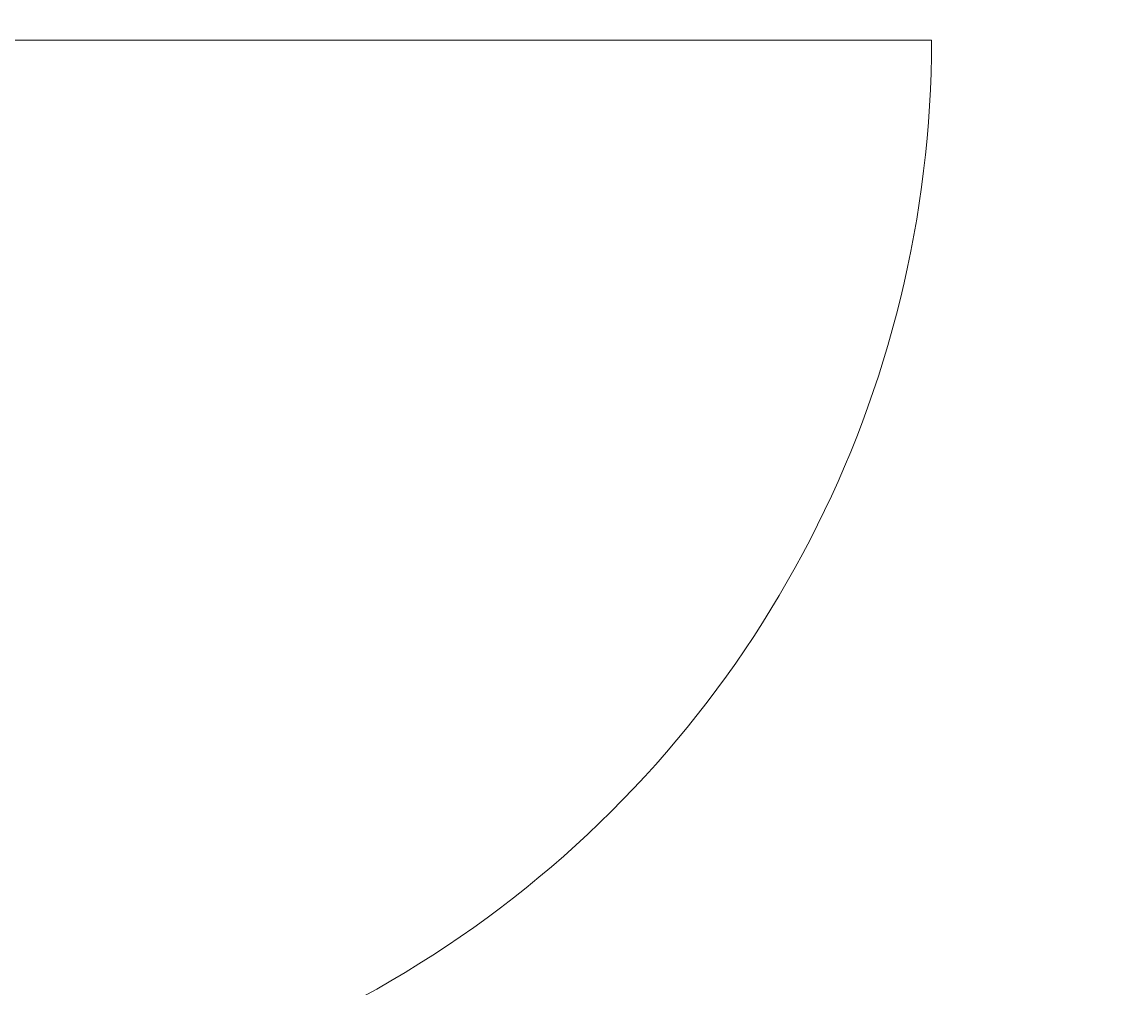
# Model space of a CAD drawing. Units: inches. Extents: x 1962 to 2771, y 1245 to 2660.
# Tile 67 of 114: x 2523 to 2551, y 2091 to 2115. Entities that reach past the tile are written whole.
import ezdxf

# ---------------------------------------------------------------- set-up
doc = ezdxf.new("R2010")
doc.units = ezdxf.units.IN
doc.layers.add('A-ANNO-DIMS', color=2, linetype='Continuous', lineweight=18)
doc.layers.add('A-DOOR', color=3, linetype='Continuous', lineweight=18)
doc.styles.get("Standard").update_dxf_attribs({"font": 'arial.ttf'})
doc.dimstyles.get("Standard").update_dxf_attribs({"dimtxt": 0.18, "dimasz": 0.18, "dimexe": 0.18, "dimexo": 0.0625, "dimgap": 0.09, "dimtad": 0, "dimtih": 1, "dimtoh": 1, "dimdec": 4, "dimzin": 0, "dimdsep": 46, "dimtxsty": 'Standard', "dimcen": 0.09, "dimadec": 0, "dimazin": 0, "dimtfac": 1, "dimtdec": 4, "dimtofl": 0, "dimtmove": 0, "dimatfit": 3, "dimfxl": 1, "dimtolj": 1, "dimtzin": 0, "dimarcsym": 0})

# ---------------------------------------------------------------- blocks, each defined once
blk = doc.blocks.new('*D40')
at = {"layer": 'A-ANNO-DIMS', "color": 0, "lineweight": -2, "transparency": 16777216}
for p, q in [((2072.02, 2033.906), (2072.02, 2583.474)), ((2660.807, 2524.406), (2660.807, 2583.474)), ((2072.2, 2583.294), (2366.02, 2583.294)), ((2660.627, 2583.294), (2366.808, 2583.294))]:
    blk.add_line(p, q, dxfattribs=at)
at = {"layer": 'A-ANNO-DIMS', "color": 0, "transparency": 16777216}
for points in [[(2072.2, 2583.324), (2072.2, 2583.264), (2072.02, 2583.294)], [(2660.627, 2583.324), (2660.627, 2583.264), (2660.807, 2583.294)]]:
    blk.add_solid(points, dxfattribs=at)
at = {"layer": 'Defpoints', "color": 0, "transparency": 16777216}
for p in [(2660.807, 2583.294), (2660.807, 2524.344), (2072.02, 2033.844)]:
    blk.add_point(p, dxfattribs=at)
at = {"layer": 'A-ANNO-DIMS', "color": 0, "transparency": 16777216, "insert": (2366.414, 2583.294), "char_height": 0.18, "attachment_point": 5}
blk.add_mtext('\\A1;588.8', dxfattribs=at)

msp = doc.modelspace()

# ---------------------------------------------------------------- linework, layer by layer
at = {"layer": 'A-DOOR'}
msp.add_line((2510.0574, 2114.3027), (2546.0574, 2114.3027), dxfattribs=at)
msp.add_arc((2518.9529, 2114.3027), 27.1044, 250.84069, 360, dxfattribs=at)

# ---------------------------------------------------------------- dimensions: what is measured, and where the dimension line sits
at = {"layer": 'A-ANNO-DIMS'}
dim = msp.add_linear_dim(base=(2660.8074, 2583.2937), p1=(2072.0204, 2033.8437), p2=(2660.8074, 2524.3437), dimstyle='Standard', override={"dimdec": 1, "dimlfac": 1, "dimrnd": 0, "dimzin": 0, "dimdsep": 46, "dimlunit": 2}, dxfattribs=at)
dim.commit()
dim.dimension.update_dxf_attribs({"geometry": '*D40', "text_midpoint": (2366.4139, 2583.2937)})

doc.saveas('drawing.dxf')
